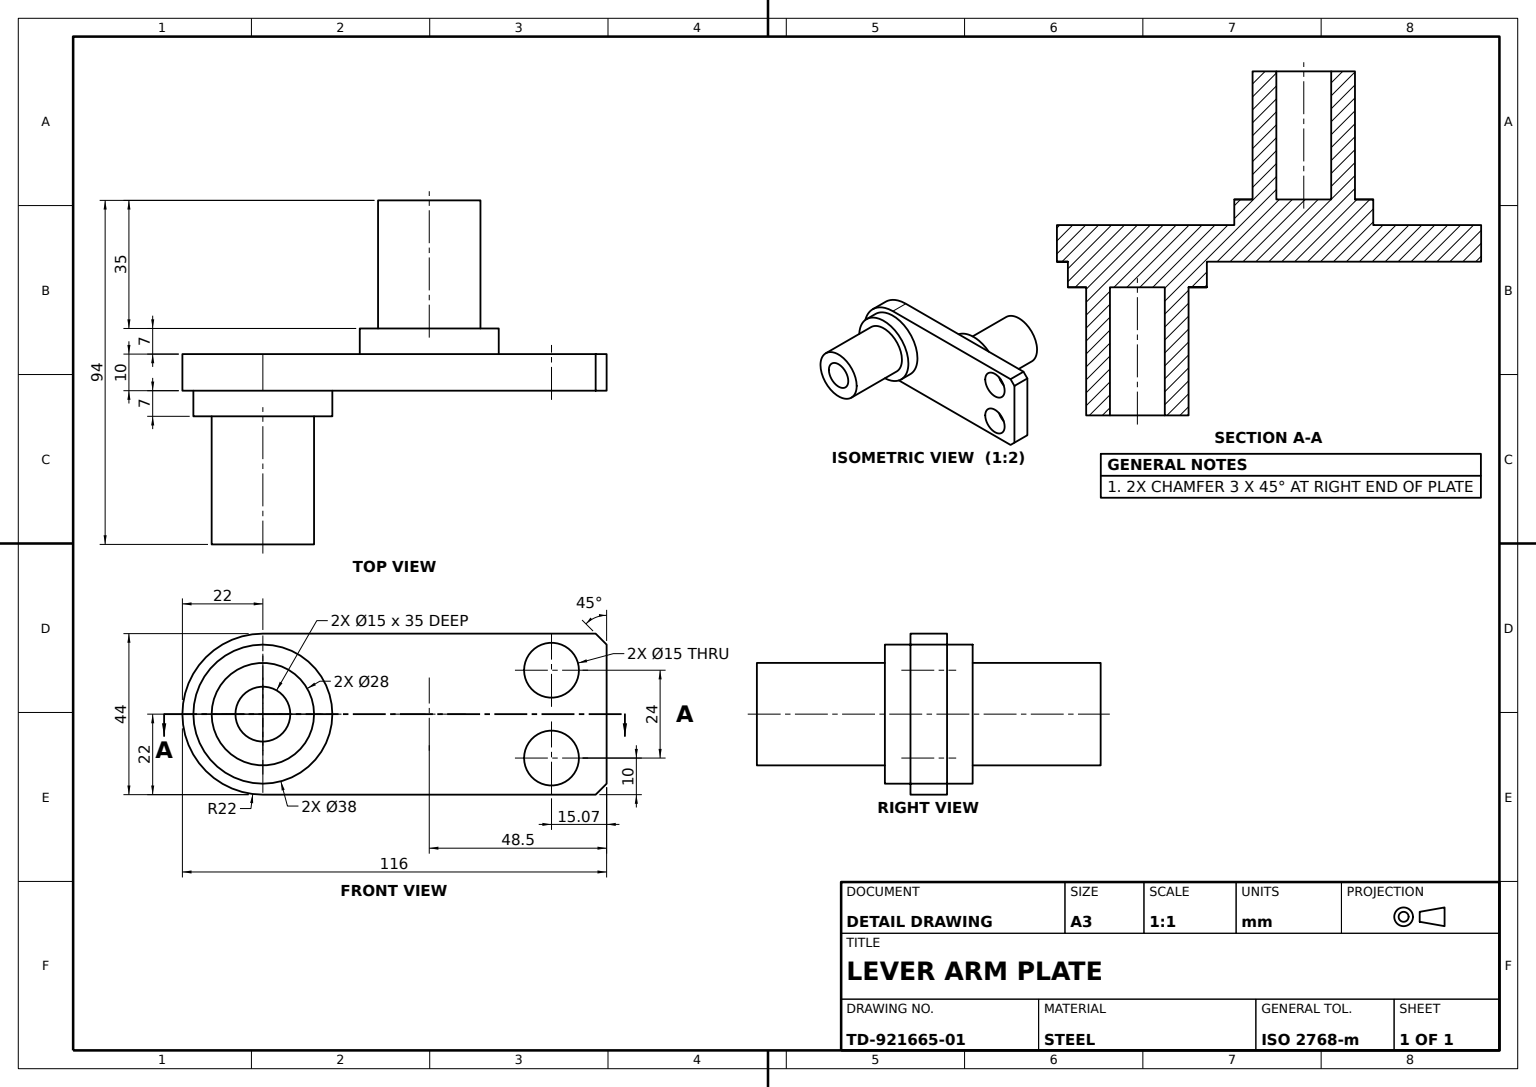
from build123d import *

# Parameters (mm, degrees)
BASE_PLATE_DEPTH      = 10
FRONT_COLLAR_SKETCH_R = 19
FRONT_COLLAR_38_DEPTH = 7
FRONT_SHAFT_SKETCH_R  = 14
FRONT_SHAFT_28_DEPTH  = 35
REAR_COLLAR_SKETCH_R  = 19
REAR_COLLAR_38_DEPTH  = 7
REAR_SHAFT_SKETCH_R   = 14
REAR_SHAFT_28_DEPTH   = 35
REAR_BORE_SKETCH_R    = 7.5
REAR_BORE_15_DEPTH    = 35
FRONT_BORE_SKETCH_R   = 7.5
FRONT_BORE_15_DEPTH   = 35
END_HOLES_SKETCH_R    = 7.5
END_HOLES_2X_15_DEPTH = 10


with BuildPart() as part:
    # Base Plate Sketch → Base Plate (new body)
    with BuildSketch(Plane.XY):
        with BuildLine():
            Line((0, 22), (69, 22))
            Line((69, 22), (91, 22))
            Line((91, 22), (94, 19))
            Line((94, 19), (94, -19))
            Line((94, -19), (91, -22))
            Line((91, -22), (69, -22))
            Line((69, -22), (0, -22))
            ThreePointArc((0, -22), (-22, 0), (0, 22))
        make_face()
    extrude(amount=BASE_PLATE_DEPTH)

    # Front Collar Sketch → Front Collar Ø38 (add)
    with BuildSketch(Plane.XY.offset(10)):
        Circle(FRONT_COLLAR_SKETCH_R)
    extrude(amount=FRONT_COLLAR_38_DEPTH)

    # Front Shaft Sketch → Front Shaft Ø28 (add)
    with BuildSketch(Plane.XY.offset(17)):
        Circle(FRONT_SHAFT_SKETCH_R)
    extrude(amount=FRONT_SHAFT_28_DEPTH)

    # Rear Collar Sketch → Rear Collar Ø38 (add)
    with BuildSketch(Plane(origin=(0, 0, 0), x_dir=(-1, 0, 0), z_dir=(0, 0, -1))):
        with Locations(Location((-45.5, 0, 0), (0, 0, 180))):
            Circle(REAR_COLLAR_SKETCH_R)
    extrude(amount=REAR_COLLAR_38_DEPTH)

    # Rear Shaft Sketch → Rear Shaft Ø28 (add)
    with BuildSketch(Plane(origin=(0, 0, -7), x_dir=(-1, 0, 0), z_dir=(0, 0, -1))):
        with Locations((-45.5, 0)):
            Circle(REAR_SHAFT_SKETCH_R)
    extrude(amount=REAR_SHAFT_28_DEPTH)

    # Rear Bore Sketch → Rear Bore Ø15 (cut)
    with BuildSketch(Plane(origin=(0, 0, -42), x_dir=(-1, 0, 0), z_dir=(0, 0, -1))):
        with Locations((-45.5, 0)):
            Circle(REAR_BORE_SKETCH_R)
    extrude(amount=-REAR_BORE_15_DEPTH, mode=Mode.SUBTRACT)

    # Front Bore Sketch → Front Bore Ø15 (cut)
    with BuildSketch(Plane.XY.offset(52)):
        Circle(FRONT_BORE_SKETCH_R)
    extrude(amount=-FRONT_BORE_15_DEPTH, mode=Mode.SUBTRACT)

    # End Holes Sketch → End Holes 2xØ15 (cut)
    with BuildSketch(Plane.XY.offset(10)):
        with Locations((78.929188111, 12)):
            Circle(END_HOLES_SKETCH_R)
        with Locations((78.929188111, -12)):
            Circle(END_HOLES_SKETCH_R)
    extrude(amount=-END_HOLES_2X_15_DEPTH, mode=Mode.SUBTRACT)


solid = part.part
